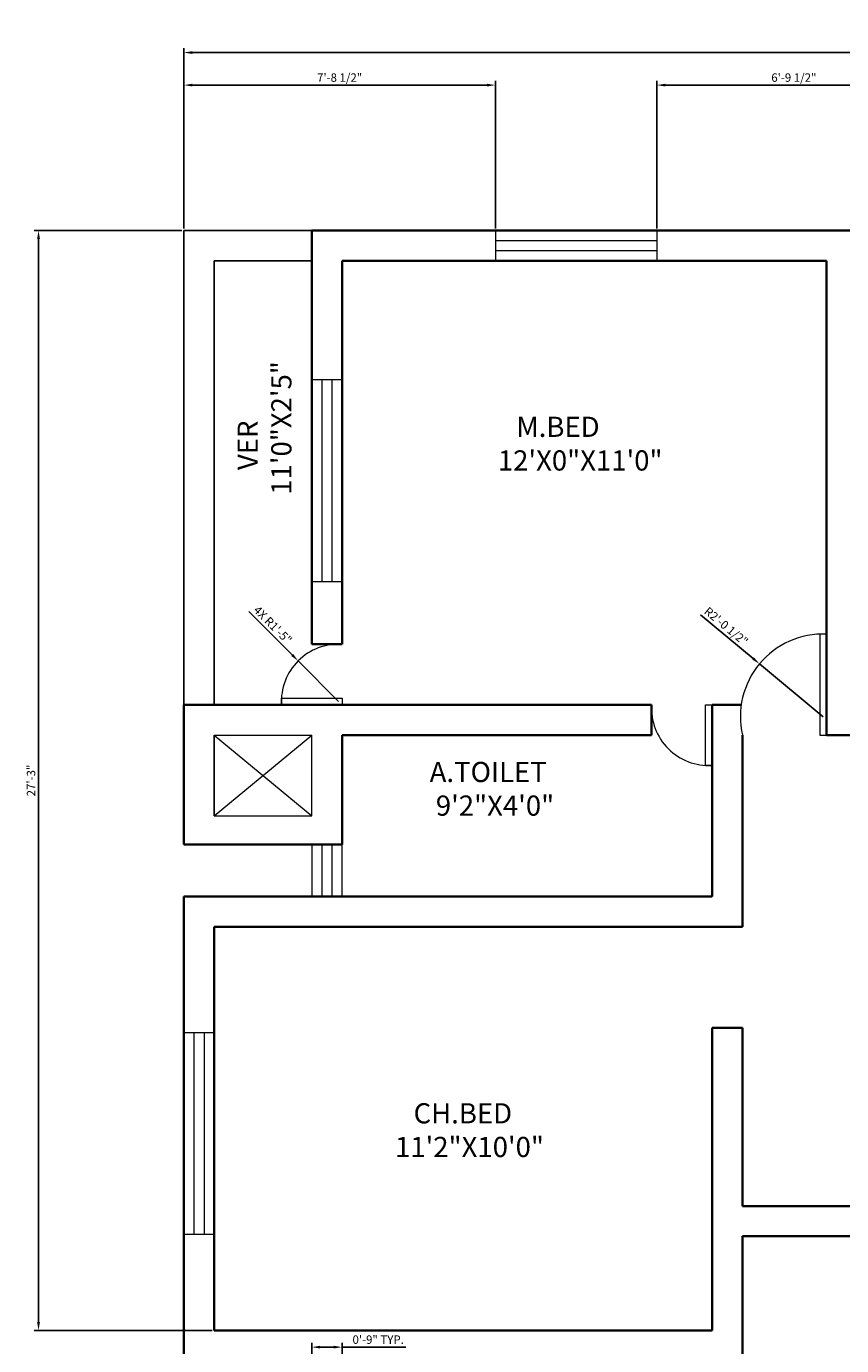
# Model space of a CAD drawing. Units: inches. Extents: x 3941 to 4852, y 2755 to 3388.
# Tile 2 of 5: x 3941 to 4184, y 2996 to 3388. Entities that reach past the tile are written whole.
import ezdxf

# ---------------------------------------------------------------- set-up
doc = ezdxf.new("R2010")
doc.units = ezdxf.units.IN
for name, color, linetype, lineweight in [('A-ANNO-DIMS', 2, 'Continuous', 18), ('A-AREA-IDEN', 7, 'Continuous', 18), ('A-DOOR', 2, 'Continuous', 18), ('A-FLOR-OPEN', 7, 'Continuous', 18), ('A-GLAZ', 5, 'Continuous', 18), ('A-WALL', 7, 'Continuous', 35), ('A-WALL-PRPT', 6, 'Continuous', 25)]:
    doc.layers.add(name, color=color, linetype=linetype, lineweight=lineweight)
doc.styles.get("Standard").update_dxf_attribs({"font": 'arial.ttf'})
doc.dimstyles.new('ISO-25', dxfattribs={"dimtxt": 2.5, "dimasz": 2.5, "dimexe": 1.25, "dimexo": 0.625, "dimtad": 1, "dimlunit": 3, "dimtxsty": 'Standard', "dimcen": 2.5, "dimadec": 0, "dimazin": 0, "dimtfac": 1, "dimtmove": 0, "dimatfit": 3, "dimfxl": 1, "dimarcsym": 0})

# ---------------------------------------------------------------- blocks, each defined once
blk = doc.blocks.new('*D1')
at = {"layer": 'A-ANNO-DIMS', "color": 0, "lineweight": -2, "transparency": 16777216}
for p, q in [((3988.25, 3328.38), (3988.25, 3381.9)), ((3990.75, 3380.65), (4801.75, 3380.65)), ((4804.25, 3328.38), (4804.25, 3381.9))]:
    blk.add_line(p, q, dxfattribs=at)
at = {"layer": 'A-ANNO-DIMS', "color": 0, "transparency": 16777216}
for points in [[(3990.75, 3381.06), (3990.75, 3380.23), (3988.25, 3380.65)], [(4801.75, 3381.06), (4801.75, 3380.23), (4804.25, 3380.65)]]:
    blk.add_solid(points, dxfattribs=at)
at = {"layer": 'Defpoints', "color": 0, "transparency": 16777216}
for p in [(4804.25, 3380.65), (3988.25, 3327.75), (4804.25, 3327.75)]:
    blk.add_point(p, dxfattribs=at)
at = {"layer": 'A-ANNO-DIMS', "color": 0, "transparency": 16777216, "insert": (4396.25, 3384.34), "char_height": 6, "attachment_point": 5}
blk.add_mtext("68'", dxfattribs=at)
blk = doc.blocks.new('WINDOW-60IN')
for p, q in [((0, 60), (9, 60)), ((0, 60), (0, 0)), ((3, 60), (3, 0)), ((6, 60), (6, 0)), ((9, 0), (9, 60)), ((0, 0), (9, 0))]:
    blk.add_line(p, q)
blk = doc.blocks.new('WINDOW-48IN')
for p, q in [((0, 9), (0, 0)), ((0, 9), (48, 9)), ((48, 9), (48, 0)), ((0, 6), (48, 6)), ((0, 3), (48, 3)), ((48, 0), (0, 0))]:
    blk.add_line(p, q)
blk = doc.blocks.new('DOOR-SWING-18IN')
for p, q in [((0.03, 0), (0.03, 2)), ((0.03, 2), (18.03, 2)), ((18.03, 0), (0.03, 0)), ((18.03, 2), (18.03, 0))]:
    blk.add_line(p, q)
blk.add_arc((17.03, 1), 17.03, 86.6335, 183.3665)
blk = doc.blocks.new('*D20')
at = {"layer": 'A-ANNO-DIMS', "color": 0, "lineweight": -2, "transparency": 16777216}
for p, q in [((4026.25, 2992.38), (4026.25, 2997.05)), ((4035.25, 2992.38), (4035.25, 2997.05)), ((4028.75, 2995.8), (4032.75, 2995.8)), ((4035.25, 2995.8), (4054.24, 2995.8))]:
    blk.add_line(p, q, dxfattribs=at)
at = {"layer": 'A-ANNO-DIMS', "color": 0, "transparency": 16777216}
for points in [[(4028.75, 2996.22), (4028.75, 2995.39), (4026.25, 2995.8)], [(4032.75, 2996.22), (4032.75, 2995.39), (4035.25, 2995.8)]]:
    blk.add_solid(points, dxfattribs=at)
at = {"layer": 'Defpoints', "color": 0, "transparency": 16777216}
for p in [(4035.25, 2995.8), (4026.25, 2991.75), (4035.25, 2991.75)]:
    blk.add_point(p, dxfattribs=at)
at = {"layer": 'A-ANNO-DIMS', "color": 0, "transparency": 16777216, "insert": (4046, 2997.71), "char_height": 2.5, "attachment_point": 5}
blk.add_mtext('0\'-9" TYP.', dxfattribs=at)
blk = doc.blocks.new('*D29')
at = {"layer": 'A-ANNO-DIMS', "color": 0, "lineweight": -2, "transparency": 16777216}
for p, q in [((3987.63, 3327.75), (3943.79, 3327.75)), ((3945.04, 3003.25), (3945.04, 3325.25)), ((3996.63, 3000.75), (3943.79, 3000.75))]:
    blk.add_line(p, q, dxfattribs=at)
at = {"layer": 'A-ANNO-DIMS', "color": 0, "transparency": 16777216}
for points in [[(3944.62, 3325.25), (3945.46, 3325.25), (3945.04, 3327.75)], [(3944.62, 3003.25), (3945.46, 3003.25), (3945.04, 3000.75)]]:
    blk.add_solid(points, dxfattribs=at)
at = {"layer": 'Defpoints', "color": 0, "transparency": 16777216}
for p in [(3945.04, 3327.75), (3988.25, 3327.75), (3997.25, 3000.75)]:
    blk.add_point(p, dxfattribs=at)
at = {"layer": 'A-ANNO-DIMS', "color": 0, "transparency": 16777216, "insert": (3943.14, 3164.25), "char_height": 2.5, "attachment_point": 5, "rotation": 90}
blk.add_mtext('27\'-3"', dxfattribs=at)
blk = doc.blocks.new('*D34')
at = {"layer": 'A-ANNO-DIMS', "color": 0, "lineweight": -2, "transparency": 16777216}
for p, q in [((3988.25, 3328.38), (3988.25, 3372.22)), ((3990.75, 3370.97), (4078.34, 3370.97)), ((4080.84, 3328.38), (4080.84, 3372.22))]:
    blk.add_line(p, q, dxfattribs=at)
at = {"layer": 'A-ANNO-DIMS', "color": 0, "transparency": 16777216}
for points in [[(3990.75, 3371.38), (3990.75, 3370.55), (3988.25, 3370.97)], [(4078.34, 3371.38), (4078.34, 3370.55), (4080.84, 3370.97)]]:
    blk.add_solid(points, dxfattribs=at)
at = {"layer": 'Defpoints', "color": 0, "transparency": 16777216}
for p in [(4080.84, 3370.97), (3988.25, 3327.75), (4080.84, 3327.75)]:
    blk.add_point(p, dxfattribs=at)
at = {"layer": 'A-ANNO-DIMS', "color": 0, "transparency": 16777216, "insert": (4034.55, 3372.88), "char_height": 2.5, "attachment_point": 5}
blk.add_mtext('7\'-8 1/2"', dxfattribs=at)
blk = doc.blocks.new('*D35')
at = {"layer": 'A-ANNO-DIMS', "color": 0, "lineweight": -2, "transparency": 16777216}
for p, q in [((4128.84, 3328.38), (4128.84, 3372.22)), ((4131.34, 3370.97), (4207.79, 3370.97)), ((4210.29, 3328.38), (4210.29, 3372.22))]:
    blk.add_line(p, q, dxfattribs=at)
at = {"layer": 'A-ANNO-DIMS', "color": 0, "transparency": 16777216}
for points in [[(4131.34, 3371.38), (4131.34, 3370.55), (4128.84, 3370.97)], [(4207.79, 3371.38), (4207.79, 3370.55), (4210.29, 3370.97)]]:
    blk.add_solid(points, dxfattribs=at)
at = {"layer": 'Defpoints', "color": 0, "transparency": 16777216}
for p in [(4210.29, 3370.97), (4128.84, 3327.75), (4210.29, 3327.75)]:
    blk.add_point(p, dxfattribs=at)
at = {"layer": 'A-ANNO-DIMS', "color": 0, "transparency": 16777216, "insert": (4169.57, 3372.88), "char_height": 2.5, "attachment_point": 5}
blk.add_mtext('6\'-9 1/2"', dxfattribs=at)
blk = doc.blocks.new('*D47')
at = {"layer": 'A-ANNO-DIMS', "color": 0, "lineweight": -2, "transparency": 16777216}
for p, q in [((4141.82, 3213.53), (4157.43, 3200.52)), ((4178.25, 3183.17), (4159.35, 3198.92))]:
    blk.add_line(p, q, dxfattribs=at)
at = {"layer": 'A-ANNO-DIMS', "color": 0, "transparency": 16777216}
blk.add_solid([(4157.7, 3200.84), (4157.17, 3200.2), (4159.35, 3198.92)], dxfattribs=at)
at = {"layer": 'Defpoints', "color": 0, "transparency": 16777216}
for p in [(4159.35, 3198.92), (4178.25, 3183.17)]:
    blk.add_point(p, dxfattribs=at)
at = {"layer": 'A-ANNO-DIMS', "color": 0, "transparency": 16777216, "insert": (4149.24, 3209.85), "char_height": 2.5, "attachment_point": 5, "rotation": 320.1936}
blk.add_mtext('R2\'-0 1/2"', dxfattribs=at)
blk = doc.blocks.new('*D48')
at = {"layer": 'A-ANNO-DIMS', "color": 0, "lineweight": -2, "transparency": 16777216}
for p, q in [((4007.53, 3214.48), (4020.44, 3201.56)), ((4034.25, 3187.75), (4022.21, 3199.8))]:
    blk.add_line(p, q, dxfattribs=at)
at = {"layer": 'A-ANNO-DIMS', "color": 0, "transparency": 16777216}
blk.add_solid([(4020.74, 3201.86), (4020.15, 3201.27), (4022.21, 3199.8)], dxfattribs=at)
at = {"layer": 'Defpoints', "color": 0, "transparency": 16777216}
for p in [(4022.21, 3199.8), (4034.25, 3187.75)]:
    blk.add_point(p, dxfattribs=at)
at = {"layer": 'A-ANNO-DIMS', "color": 0, "transparency": 16777216, "insert": (4014.45, 3210.25), "char_height": 2.5, "attachment_point": 5, "rotation": 314.9999}
blk.add_mtext('4X R1\'-5"', dxfattribs=at)

msp = doc.modelspace()

# ---------------------------------------------------------------- linework, layer by layer
at = {"layer": 'A-DOOR'}
for p, q in [((4179.254, 3207.754), (4177.254, 3207.754)), ((4177.254, 3207.754), (4177.254, 3177.754)), ((4179.254, 3177.754), (4179.254, 3207.754)), ((4177.254, 3177.754), (4179.254, 3177.754))]:
    msp.add_line(p, q, dxfattribs=at)
msp.add_arc((4178.254, 3183.171), 24.604, 87.67061, 192.71825, dxfattribs=at)
at = {"layer": 'A-FLOR-OPEN'}
for p, q in [((3997.254, 3177.754), (4026.254, 3177.754)), ((3997.254, 3153.754), (3997.254, 3177.754)), ((3997.254, 3177.754), (3997.254, 3153.754)), ((3997.254, 3153.754), (4026.254, 3177.754)), ((3997.254, 3177.754), (3997.254, 3177.754)), ((3997.254, 3177.754), (4026.254, 3153.754)), ((4026.254, 3153.754), (4026.254, 3177.754)), ((3997.254, 3153.754), (4026.254, 3153.754))]:
    msp.add_line(p, q, dxfattribs=at)
at = {"layer": 'A-GLAZ'}
for p, q in [((4026.254, 3283.436), (4026.254, 3283.436)), ((4035.254, 3145.27), (4026.254, 3145.27)), ((4026.254, 3145.27), (4026.254, 3129.754)), ((4029.254, 3145.27), (4029.254, 3129.754)), ((4032.254, 3145.27), (4032.254, 3129.754)), ((4035.254, 3129.754), (4035.254, 3145.27)), ((4026.254, 3129.754), (4035.254, 3129.754))]:
    msp.add_line(p, q, dxfattribs=at)
at = {"layer": 'A-WALL'}
for p, q in [((4026.254, 3327.754), (4766.254, 3327.754)), ((4026.254, 3204.754), (4026.254, 3327.754)), ((4035.254, 3318.754), (4179.254, 3318.754)), ((4035.254, 3204.754), (4035.254, 3318.754)), ((4179.254, 3177.754), (4179.254, 3318.754)), ((4026.254, 3204.754), (4035.254, 3204.754)), ((3988.254, 3186.754), (4035.254, 3186.754)), ((3988.254, 3149.399), (3988.254, 3186.754)), ((4035.254, 3186.754), (4127.254, 3186.754)), ((4127.254, 3177.754), (4127.254, 3186.754)), ((4145.254, 3129.754), (4145.254, 3186.754)), ((4145.254, 3186.754), (4153.912, 3186.754)), ((4035.254, 3149.399), (4035.254, 3177.754)), ((4035.254, 3177.754), (4127.254, 3177.754)), ((4154.254, 3120.754), (4154.254, 3177.754)), ((4179.254, 3177.754), (4188.254, 3177.754)), ((3988.254, 3149.399), (3988.254, 3145.27)), ((4035.254, 3145.27), (4035.254, 3149.399)), ((3988.254, 3145.27), (4035.254, 3145.27)), ((3988.254, 3129.754), (4145.254, 3129.754)), ((3988.254, 2991.754), (3988.254, 3129.754)), ((3997.254, 3120.754), (4154.254, 3120.754)), ((3997.254, 3000.754), (3997.254, 3120.754)), ((4145.254, 3000.754), (4145.254, 3090.754)), ((4145.254, 3090.754), (4154.254, 3090.754)), ((4154.254, 3037.754), (4154.254, 3090.754)), ((4301.254, 3037.754), (4154.254, 3037.754)), ((4154.254, 2931.754), (4154.254, 3028.754)), ((4310.254, 3028.754), (4154.254, 3028.754)), ((3997.254, 3000.754), (4145.254, 3000.754))]:
    msp.add_line(p, q, dxfattribs=at)
at = {"layer": 'A-WALL-PRPT'}
for p, q in [((3988.254, 3186.754), (3988.254, 3327.754)), ((3988.254, 3327.754), (4026.254, 3327.754)), ((3997.254, 3318.754), (4026.254, 3318.754)), ((3997.254, 3186.754), (3997.254, 3318.754))]:
    msp.add_line(p, q, dxfattribs=at)

# ---------------------------------------------------------------- block references
at = {"layer": 'A-DOOR'}
msp.add_blockref('DOOR-SWING-18IN', (4017.224, 3186.754), dxfattribs=at)
at = {"layer": 'A-DOOR', "rotation": 90}
msp.add_blockref('DOOR-SWING-18IN', (4145.254, 3168.725), dxfattribs=at)
at = {"layer": 'A-GLAZ'}
for name, p in [('WINDOW-48IN', (4080.838, 3318.754)), ('WINDOW-60IN', (4026.254, 3223.436)), ('WINDOW-60IN', (3988.254, 3029.341))]:
    msp.add_blockref(name, p, dxfattribs=at)

# ---------------------------------------------------------------- texts
at = {"layer": 'A-AREA-IDEN', "insert": (4004.225, 3249.196), "char_height": 6, "attachment_point": 1, "rotation": 90}
msp.add_mtext_dynamic_manual_height_columns('    VER\\P11\'0"X2\'5"', width=69.57529, gutter_width=12.5, heights=[0], dxfattribs=at)
at = {"layer": 'A-AREA-IDEN', "char_height": 6, "attachment_point": 1}
for s, insert in [('   M.BED\\P12\'X0"X11\'0"', (4081.575, 3272.392)), ('A.TOILET\\P 9\'2"X4\'0"', (4061.307, 3169.787)), ('   CH.BED\\P11\'2"X10\'0"', (4051.02, 3068.316))]:
    msp.add_mtext_dynamic_manual_height_columns(s, width=69.57529, gutter_width=12.5, heights=[0], dxfattribs=dict(at, insert=insert))

# ---------------------------------------------------------------- dimensions: what is measured, and where the dimension line sits
at = {"layer": 'A-ANNO-DIMS'}
for base, p1, p2, override, picture, middle in [((4804.254, 3380.647), (3988.254, 3327.754), (4804.254, 3327.754), {"dimtxt": 6, "dimclrd": 0, "dimclre": 0, "dimclrt": 0}, '*D1', (4396.254, 3384.335)), ((4080.838, 3370.967), (3988.254, 3327.754), (4080.838, 3327.754), {"dimdec": 1, "dimlfac": 1, "dimrnd": 0, "dimzin": 1, "dimdsep": 46, "dimlunit": 4, "dimfrac": 2}, '*D34', (4034.546, 3372.884)), ((4210.294, 3370.967), (4128.838, 3327.754), (4210.294, 3327.754), {"dimdec": 1, "dimlfac": 1, "dimrnd": 0, "dimzin": 1, "dimdsep": 46, "dimlunit": 4, "dimfrac": 2}, '*D35', (4169.566, 3372.884))]:
    dim = msp.add_linear_dim(base=base, p1=p1, p2=p2, dimstyle='ISO-25', override=override, dxfattribs=at)
    dim.commit()
    dim.dimension.update_dxf_attribs({"geometry": picture, "text_midpoint": middle})
dim = msp.add_linear_dim(base=(3945.041, 3327.754), p1=(3997.254, 3000.754), p2=(3988.254, 3327.754), angle=90, dimstyle='ISO-25', override={"dimdec": 1, "dimlfac": 1, "dimrnd": 0, "dimzin": 1, "dimdsep": 46, "dimlunit": 4, "dimfrac": 2}, dxfattribs=at)
dim.commit()
dim.dimension.update_dxf_attribs({"geometry": '*D29', "text_midpoint": (3943.139, 3164.254)})
dim = msp.add_radius_dim(center=(4034.254, 3187.754), mpoint=(4022.212, 3199.796), text='4X <>', dimstyle='ISO-25', override={"dimdec": 1, "dimlfac": 1, "dimrnd": 0, "dimzin": 1, "dimdsep": 46, "dimlunit": 4, "dimfrac": 2}, dxfattribs=at)
dim.commit()
dim.dimension.update_dxf_attribs({"geometry": '*D48', "text_midpoint": (4014.449, 3210.248)})
dim = msp.add_radius_dim(center=(4178.254, 3183.171), mpoint=(4159.353, 3198.922), dimstyle='ISO-25', override={"dimdec": 1, "dimlfac": 1, "dimrnd": 0, "dimzin": 1, "dimdsep": 46, "dimlunit": 4, "dimfrac": 2}, dxfattribs=at)
dim.commit()
dim.dimension.update_dxf_attribs({"geometry": '*D47', "text_midpoint": (4148.012, 3208.373), "dimtype": 164})
dim = msp.add_linear_dim(base=(4035.254, 2995.804), p1=(4026.254, 2991.754), p2=(4035.254, 2991.754), text='<> TYP.', dimstyle='ISO-25', override={"dimdec": 1, "dimlfac": 1, "dimrnd": 0, "dimzin": 1, "dimdsep": 46, "dimlunit": 4, "dimfrac": 2}, dxfattribs=at)
dim.commit()
dim.dimension.update_dxf_attribs({"geometry": '*D20', "text_midpoint": (4045.998, 2997.706)})

doc.saveas('drawing.dxf')
